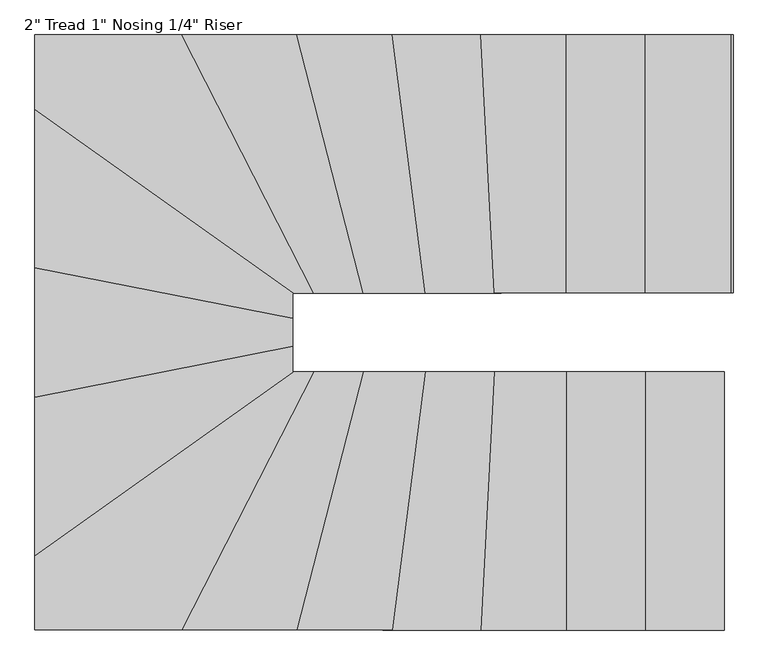
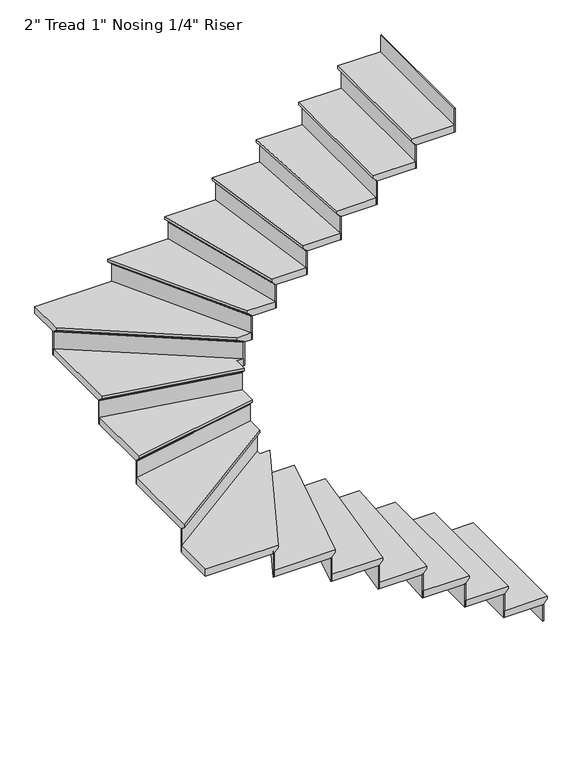
"""IFC4 building model written with IfcOpenShell, lengths in millimetres: stair flight geometry."""

from ifc_helpers import new_model, si_unit, origin, place, context, project, spatial, faceted_brep, source, transform, mapped, element, save


def stair_flight_a924437b(model_context):
    return source(origin(), model_context, "Body", "Brep", [
        faceted_brep([(-7708.0614906, -9206.110779, 6863.0131579), (-7708.0614906, -9206.110779, 6882.0631579), (-7708.0614906, -10120.510779, 6882.0631579), (-7708.0614906, -10120.510779, 6863.0131579), (-7733.4614906, -9206.110779, 6837.6131579), (-7733.4614906, -10120.510779, 6837.6131579), (-8012.8614906, -9206.110779, 6882.0631579), (-8012.8614906, -10120.510779, 6882.0631579), (-7733.4614906, -10120.510779, 6831.2631579), (-8012.8614906, -10120.510779, 6831.2631579), (-8012.8614906, -9206.110779, 6831.2631579), (-7733.4614906, -9206.110779, 6831.2631579)], [[[0, 1, 2, 3]], [[4, 0, 3, 5]], [[2, 1, 6, 7]], [[8, 9, 10, 11]], [[2, 7, 9, 8, 5, 3]], [[8, 11, 4, 5]], [[6, 1, 0, 4, 11, 10]], [[7, 6, 10, 9]]]),
        faceted_brep([(-7733.4614906, -9206.110779, 6831.2631579), (-7733.4614906, -9206.110779, 6705.6), (-7739.8114906, -9206.110779, 6705.6), (-7739.8114906, -9206.110779, 6831.2631579), (-7733.4614906, -10120.510779, 6831.2631579), (-7739.8114906, -10120.510779, 6831.2631579), (-7739.8114906, -10120.510779, 6705.6), (-7733.4614906, -10120.510779, 6705.6)], [[[0, 1, 2, 3]], [[4, 5, 6, 7]], [[1, 0, 4, 7]], [[2, 1, 7, 6]], [[3, 2, 6, 5]], [[0, 3, 5, 4]]]),
        faceted_brep([(-8012.8614906, -9206.110779, 7007.7263158), (-8012.8614906, -9206.110779, 6831.2631579), (-8019.2114906, -9206.110779, 6831.2631579), (-8019.2114906, -9206.110779, 7007.7263158), (-8012.8614906, -10120.510779, 7007.7263158), (-8019.2114906, -10120.510779, 7007.7263158), (-8019.2114906, -10120.510779, 6831.2631579), (-8012.8614906, -10120.510779, 6831.2631579)], [[[0, 1, 2, 3]], [[4, 5, 6, 7]], [[1, 0, 4, 7]], [[2, 1, 7, 6]], [[3, 2, 6, 5]], [[0, 3, 5, 4]]]),
        faceted_brep([(-7987.4614906, -10120.510779, 7058.5263158), (-7987.4614906, -9206.110779, 7058.5263158), (-8292.2614906, -9206.110779, 7058.5263158), (-8292.2614906, -10120.510779, 7058.5263158), (-8012.8614906, -10120.510779, 7007.7263158), (-8292.2614906, -10120.510779, 7007.7263158), (-8292.2614906, -9206.110779, 7007.7263158), (-8012.8614906, -9206.110779, 7007.7263158), (-8012.8614906, -10120.510779, 7014.0763158), (-7987.4614906, -10120.510779, 7039.4763158), (-8012.8614906, -9206.110779, 7014.0763158), (-7987.4614906, -9206.110779, 7039.4763158)], [[[0, 1, 2, 3]], [[4, 5, 6, 7]], [[0, 3, 5, 4, 8, 9]], [[4, 7, 10, 8]], [[2, 1, 11, 10, 7, 6]], [[3, 2, 6, 5]], [[11, 1, 0, 9]], [[10, 11, 9, 8]]]),
        faceted_brep([(-8292.2614906, -9206.110779, 7184.1894737), (-8292.2614906, -9206.110779, 7007.7263158), (-8298.6114906, -9206.110779, 7007.7263158), (-8298.6114906, -9206.110779, 7184.1894737), (-8292.2614906, -10120.510779, 7184.1894737), (-8298.6114906, -10120.510779, 7184.1894737), (-8298.6114906, -10120.510779, 7007.7263158), (-8292.2614906, -10120.510779, 7007.7263158)], [[[0, 1, 2, 3]], [[4, 5, 6, 7]], [[1, 0, 4, 7]], [[2, 1, 7, 6]], [[3, 2, 6, 5]], [[0, 3, 5, 4]]]),
        faceted_brep([(-8266.8614906, -10120.510779, 7234.9894737), (-8266.8614906, -9206.110779, 7234.9894737), (-8547.928652, -9206.110779, 7234.9894737), (-8595.4629224, -10120.510779, 7234.9894737), (-8292.2614906, -10120.510779, 7184.1894737), (-8595.4629224, -10120.510779, 7184.1894737), (-8547.928652, -9206.110779, 7184.1894737), (-8292.2614906, -9206.110779, 7184.1894737), (-8292.2614906, -10120.510779, 7190.5394737), (-8266.8614906, -10120.510779, 7215.9394737), (-8292.2614906, -9206.110779, 7190.5394737), (-8266.8614906, -9206.110779, 7215.9394737)], [[[0, 1, 2, 3]], [[4, 5, 6, 7]], [[0, 3, 5, 4, 8, 9]], [[4, 7, 10, 8]], [[2, 1, 11, 10, 7, 6]], [[3, 2, 6, 5]], [[11, 1, 0, 9]], [[10, 11, 9, 8]]]),
        faceted_brep([(-8547.928652, -9206.110779, 7360.6526316), (-8547.928652, -9206.110779, 7184.1894737), (-8554.2872262, -9206.110779, 7184.1894737), (-8554.2872262, -9206.110779, 7360.6526316), (-8595.4629224, -10120.510779, 7360.6526316), (-8601.8214966, -10120.510779, 7360.6526316), (-8601.8214966, -10120.510779, 7184.1894737), (-8595.4629224, -10120.510779, 7184.1894737)], [[[0, 1, 2, 3]], [[4, 5, 6, 7]], [[1, 0, 4, 7]], [[2, 1, 7, 6]], [[3, 2, 6, 5]], [[0, 3, 5, 4]]]),
        faceted_brep([(-8570.0286258, -10120.510779, 7411.4526316), (-8522.4943554, -9206.110779, 7411.4526316), (-8792.0953519, -9206.110779, 7411.4526316), (-8910.4514035, -10120.510779, 7411.4526316), (-8595.4629224, -10120.510779, 7360.6526316), (-8910.4514035, -10120.510779, 7360.6526316), (-8792.0953519, -9206.110779, 7360.6526316), (-8547.928652, -9206.110779, 7360.6526316), (-8595.4629224, -10120.510779, 7367.0026316), (-8570.0286258, -10120.510779, 7392.4026316), (-8547.928652, -9206.110779, 7367.0026316), (-8522.4943554, -9206.110779, 7392.4026316)], [[[0, 1, 2, 3]], [[4, 5, 6, 7]], [[0, 3, 5, 4, 8, 9]], [[4, 7, 10, 8]], [[2, 1, 11, 10, 7, 6]], [[3, 2, 6, 5]], [[11, 1, 0, 9]], [[10, 11, 9, 8]]]),
        faceted_brep([(-8792.0953519, -9206.110779, 7537.1157895), (-8792.0953519, -9206.110779, 7360.6526316), (-8798.4983236, -9206.110779, 7360.6526316), (-8798.4983236, -9206.110779, 7537.1157895), (-8910.4514035, -10120.510779, 7537.1157895), (-8916.8543753, -10120.510779, 7537.1157895), (-8916.8543753, -10120.510779, 7360.6526316), (-8910.4514035, -10120.510779, 7360.6526316)], [[[0, 1, 2, 3]], [[4, 5, 6, 7]], [[1, 0, 4, 7]], [[2, 1, 7, 6]], [[3, 2, 6, 5]], [[0, 3, 5, 4]]]),
        faceted_brep([(-8884.8395164, -10120.510779, 7587.9157895), (-8766.4834647, -9206.110779, 7587.9157895), (-9013.7225743, -9206.110779, 7587.9157895), (-9248.8530217, -10120.510779, 7587.9157895), (-8910.4514035, -10120.510779, 7537.1157895), (-9248.8530217, -10120.510779, 7537.1157895), (-9013.7225743, -9206.110779, 7537.1157895), (-8792.0953519, -9206.110779, 7537.1157895), (-8910.4514035, -10120.510779, 7543.4657895), (-8884.8395164, -10120.510779, 7568.8657895), (-8792.0953519, -9206.110779, 7543.4657895), (-8766.4834647, -9206.110779, 7568.8657895)], [[[0, 1, 2, 3]], [[4, 5, 6, 7]], [[0, 3, 5, 4, 8, 9]], [[4, 7, 10, 8]], [[2, 1, 11, 10, 7, 6]], [[3, 2, 6, 5]], [[11, 1, 0, 9]], [[10, 11, 9, 8]]]),
        faceted_brep([(-9013.7225743, -9206.110779, 7713.5789474), (-9013.7225743, -9206.110779, 7537.1157895), (-9020.2791512, -9206.110779, 7537.1157895), (-9020.2791512, -9206.110779, 7713.5789474), (-9248.8530217, -10120.510779, 7713.5789474), (-9255.4095986, -10120.510779, 7713.5789474), (-9255.4095986, -10120.510779, 7537.1157895), (-9248.8530217, -10120.510779, 7537.1157895)], [[[0, 1, 2, 3]], [[4, 5, 6, 7]], [[1, 0, 4, 7]], [[2, 1, 7, 6]], [[3, 2, 6, 5]], [[0, 3, 5, 4]]]),
        faceted_brep([(-9222.6267143, -10120.510779, 7764.3789474), (-8987.4962669, -9206.110779, 7764.3789474), (-9190.0692104, -9206.110779, 7764.3789474), (-9658.8938317, -10120.510779, 7764.3789474), (-9248.8530217, -10120.510779, 7713.5789474), (-9658.8938317, -10120.510779, 7713.5789474), (-9190.0692104, -9206.110779, 7713.5789474), (-9013.7225743, -9206.110779, 7713.5789474), (-9248.8530217, -10120.510779, 7719.9289474), (-9222.6267143, -10120.510779, 7745.3289474), (-9013.7225743, -9206.110779, 7719.9289474), (-8987.4962669, -9206.110779, 7745.3289474)], [[[0, 1, 2, 3]], [[4, 5, 6, 7]], [[0, 3, 5, 4, 8, 9]], [[4, 7, 10, 8]], [[2, 1, 11, 10, 7, 6]], [[3, 2, 6, 5]], [[11, 1, 0, 9]], [[10, 11, 9, 8]]]),
        faceted_brep([(-9190.0692104, -9206.110779, 7890.0421053), (-9190.0692104, -9206.110779, 7713.5789474), (-9197.2051936, -9206.110779, 7713.5789474), (-9197.2051936, -9206.110779, 7890.0421053), (-9658.8938317, -10120.510779, 7890.0421053), (-9666.0298149, -10120.510779, 7890.0421053), (-9666.0298149, -10120.510779, 7713.5789474), (-9658.8938317, -10120.510779, 7713.5789474)], [[[0, 1, 2, 3]], [[4, 5, 6, 7]], [[1, 0, 4, 7]], [[2, 1, 7, 6]], [[3, 2, 6, 5]], [[0, 3, 5, 4]]]),
        faceted_brep([(-10150.1931824, -9826.8296453, 7940.8421053), (-10150.1931824, -10120.510779, 7940.8421053), (-9630.3498992, -10120.510779, 7940.8421053), (-9161.5252779, -9206.110779, 7940.8421053), (-9235.7931824, -9206.110779, 7940.8421053), (-9235.7931824, -9176.5556961, 7940.8421053), (-10150.1931824, -10120.510779, 7890.0421053), (-10150.1931824, -9826.8296453, 7890.0421053), (-9235.7931824, -9176.5556961, 7890.0421053), (-9235.7931824, -9206.110779, 7890.0421053), (-9190.0692104, -9206.110779, 7890.0421053), (-9658.8938317, -10120.510779, 7890.0421053), (-9658.8938317, -10120.510779, 7896.3921053), (-9630.3498992, -10120.510779, 7921.7921053), (-9190.0692104, -9206.110779, 7896.3921053), (-9161.5252779, -9206.110779, 7921.7921053)], [[[0, 1, 2, 3, 4, 5]], [[6, 7, 8, 9, 10, 11]], [[1, 0, 7, 6]], [[2, 1, 6, 11, 12, 13]], [[11, 10, 14, 12]], [[4, 3, 15, 14, 10, 9]], [[5, 4, 9, 8]], [[0, 5, 8, 7]], [[15, 3, 2, 13]], [[14, 15, 13, 12]]]),
        faceted_brep([(-9235.7931824, -9176.5556961, 8066.5052632), (-9235.7931824, -9176.5556961, 7890.0421053), (-9235.7931824, -9168.7637213, 7890.0421053), (-9235.7931824, -9168.7637213, 8066.5052632), (-10150.1931824, -9826.8296453, 8066.5052632), (-10150.1931824, -9819.0376705, 8066.5052632), (-10150.1931824, -9819.0376705, 7890.0421053), (-10150.1931824, -9826.8296453, 7890.0421053)], [[[0, 1, 2, 3]], [[4, 5, 6, 7]], [[1, 0, 4, 7]], [[2, 1, 7, 6]], [[3, 2, 6, 5]], [[0, 3, 5, 4]]]),
        faceted_brep([(-10150.1931824, -9857.9975445, 8117.3052632), (-9235.7931824, -9207.7235953, 8117.3052632), (-9235.7931824, -9090.1016091, 8117.3052632), (-10150.1931824, -9270.3424654, 8117.3052632), (-10150.1931824, -9826.8296453, 8066.5052632), (-10150.1931824, -9270.3424654, 8066.5052632), (-9235.7931824, -9090.1016091, 8066.5052632), (-9235.7931824, -9176.5556961, 8066.5052632), (-10150.1931824, -9826.8296453, 8072.8552632), (-10150.1931824, -9857.9975445, 8098.2552632), (-9235.7931824, -9176.5556961, 8072.8552632), (-9235.7931824, -9207.7235953, 8098.2552632)], [[[0, 1, 2, 3]], [[4, 5, 6, 7]], [[0, 3, 5, 4, 8, 9]], [[4, 7, 10, 8]], [[2, 1, 11, 10, 7, 6]], [[3, 2, 6, 5]], [[11, 1, 0, 9]], [[10, 11, 9, 8]]]),
        faceted_brep([(-9235.7931824, -9090.1016091, 8242.9684211), (-9235.7931824, -9090.1016091, 8066.5052632), (-9235.7931824, -9083.6294236, 8066.5052632), (-9235.7931824, -9083.6294236, 8242.9684211), (-10150.1931824, -9270.3424654, 8242.9684211), (-10150.1931824, -9263.87028, 8242.9684211), (-10150.1931824, -9263.87028, 8066.5052632), (-10150.1931824, -9270.3424654, 8066.5052632)], [[[0, 1, 2, 3]], [[4, 5, 6, 7]], [[1, 0, 4, 7]], [[2, 1, 7, 6]], [[3, 2, 6, 5]], [[0, 3, 5, 4]]]),
        faceted_brep([(-10150.1931824, -9296.2312071, 8293.7684211), (-9235.7931824, -9115.9903508, 8293.7684211), (-9235.7931824, -8990.9424654, 8293.7684211), (-10150.1931824, -8810.7016091, 8293.7684211), (-10150.1931824, -9270.3424654, 8242.9684211), (-10150.1931824, -8810.7016091, 8242.9684211), (-9235.7931824, -8990.9424654, 8242.9684211), (-9235.7931824, -9090.1016091, 8242.9684211), (-10150.1931824, -9270.3424654, 8249.3184211), (-10150.1931824, -9296.2312071, 8274.7184211), (-9235.7931824, -9090.1016091, 8249.3184211), (-9235.7931824, -9115.9903508, 8274.7184211)], [[[0, 1, 2, 3]], [[4, 5, 6, 7]], [[0, 3, 5, 4, 8, 9]], [[4, 7, 10, 8]], [[2, 1, 11, 10, 7, 6]], [[3, 2, 6, 5]], [[11, 1, 0, 9]], [[10, 11, 9, 8]]]),
        faceted_brep([(-9235.7931824, -8990.9424654, 8419.4315789), (-9235.7931824, -8990.9424654, 8242.9684211), (-9235.7931824, -8984.47028, 8242.9684211), (-9235.7931824, -8984.47028, 8419.4315789), (-10150.1931824, -8810.7016091, 8419.4315789), (-10150.1931824, -8804.2294236, 8419.4315789), (-10150.1931824, -8804.2294236, 8242.9684211), (-10150.1931824, -8810.7016091, 8242.9684211)], [[[0, 1, 2, 3]], [[4, 5, 6, 7]], [[1, 0, 4, 7]], [[2, 1, 7, 6]], [[3, 2, 6, 5]], [[0, 3, 5, 4]]]),
        faceted_brep([(-10150.1931824, -8836.5903508, 8470.2315789), (-9235.7931824, -9016.8312071, 8470.2315789), (-9235.7931824, -8926.710779, 8470.2315789), (-9189.6977079, -8926.710779, 8470.2315789), (-10150.1931824, -8243.6561143, 8470.2315789), (-10150.1931824, -8810.7016091, 8419.4315789), (-10150.1931824, -8243.6561143, 8419.4315789), (-9189.6977079, -8926.710779, 8419.4315789), (-9235.7931824, -8926.710779, 8419.4315789), (-9235.7931824, -8990.9424654, 8419.4315789), (-10150.1931824, -8810.7016091, 8425.7815789), (-10150.1931824, -8836.5903508, 8451.1815789), (-9235.7931824, -8990.9424654, 8425.7815789), (-9235.7931824, -9016.8312071, 8451.1815789)], [[[0, 1, 2, 3, 4]], [[5, 6, 7, 8, 9]], [[0, 4, 6, 5, 10, 11]], [[5, 9, 12, 10]], [[2, 1, 13, 12, 9, 8]], [[3, 2, 8, 7]], [[4, 3, 7, 6]], [[13, 1, 0, 11]], [[12, 13, 11, 10]]]),
        faceted_brep([(-9189.6977079, -8926.710779, 8595.8947368), (-9189.6977079, -8926.710779, 8419.4315789), (-9178.7408154, -8926.710779, 8419.4315789), (-9178.7408154, -8926.710779, 8595.8947368), (-10150.1931824, -8243.6561143, 8595.8947368), (-10150.1931824, -8235.8641395, 8595.8947368), (-10150.1931824, -8235.8641395, 8419.4315789), (-10150.1931824, -8243.6561143, 8419.4315789)], [[[0, 1, 2, 3]], [[4, 5, 6, 7]], [[1, 0, 4, 7]], [[2, 1, 7, 6]], [[3, 2, 6, 5]], [[0, 3, 5, 4]]]),
        faceted_brep([(-9601.8059667, -8012.310779, 8646.6947368), (-10150.1931824, -8012.310779, 8646.6947368), (-10150.1931824, -8274.8240135, 8646.6947368), (-9233.5252779, -8926.710779, 8646.6947368), (-9132.9813454, -8926.710779, 8646.6947368), (-10150.1931824, -8012.310779, 8595.8947368), (-9601.8059667, -8012.310779, 8595.8947368), (-9132.9813454, -8926.710779, 8595.8947368), (-9189.6977079, -8926.710779, 8595.8947368), (-10150.1931824, -8243.6561143, 8595.8947368), (-10150.1931824, -8243.6561143, 8602.2447368), (-10150.1931824, -8274.8240135, 8627.6447368), (-9189.6977079, -8926.710779, 8602.2447368), (-9233.5252779, -8926.710779, 8627.6447368)], [[[0, 1, 2, 3, 4]], [[5, 6, 7, 8, 9]], [[1, 0, 6, 5]], [[2, 1, 5, 9, 10, 11]], [[9, 8, 12, 10]], [[4, 3, 13, 12, 8, 7]], [[0, 4, 7, 6]], [[13, 3, 2, 11]], [[12, 13, 11, 10]]]),
        faceted_brep([(-9132.9813454, -8926.710779, 8772.3578947), (-9132.9813454, -8926.710779, 8595.8947368), (-9125.8453622, -8926.710779, 8595.8947368), (-9125.8453622, -8926.710779, 8772.3578947), (-9601.8059667, -8012.310779, 8772.3578947), (-9594.6699835, -8012.310779, 8772.3578947), (-9594.6699835, -8012.310779, 8595.8947368), (-9601.8059667, -8012.310779, 8595.8947368)], [[[0, 1, 2, 3]], [[4, 5, 6, 7]], [[1, 0, 4, 7]], [[2, 1, 7, 6]], [[3, 2, 6, 5]], [[0, 3, 5, 4]]]),
        faceted_brep([(-9630.3498992, -8012.310779, 8823.1578947), (-9161.5252779, -8926.710779, 8823.1578947), (-8961.2699594, -8926.710779, 8823.1578947), (-9196.4004068, -8012.310779, 8823.1578947), (-9601.8059667, -8012.310779, 8772.3578947), (-9196.4004068, -8012.310779, 8772.3578947), (-8961.2699594, -8926.710779, 8772.3578947), (-9132.9813454, -8926.710779, 8772.3578947), (-9601.8059667, -8012.310779, 8778.7078947), (-9630.3498992, -8012.310779, 8804.1078947), (-9132.9813454, -8926.710779, 8778.7078947), (-9161.5252779, -8926.710779, 8804.1078947)], [[[0, 1, 2, 3]], [[4, 5, 6, 7]], [[0, 3, 5, 4, 8, 9]], [[4, 7, 10, 8]], [[2, 1, 11, 10, 7, 6]], [[3, 2, 6, 5]], [[11, 1, 0, 9]], [[10, 11, 9, 8]]]),
        faceted_brep([(-8961.2699594, -8926.710779, 8948.8210526), (-8961.2699594, -8926.710779, 8772.3578947), (-8954.7133825, -8926.710779, 8772.3578947), (-8954.7133825, -8926.710779, 8948.8210526), (-9196.4004068, -8012.310779, 8948.8210526), (-9189.84383, -8012.310779, 8948.8210526), (-9189.84383, -8012.310779, 8772.3578947), (-9196.4004068, -8012.310779, 8772.3578947)], [[[0, 1, 2, 3]], [[4, 5, 6, 7]], [[1, 0, 4, 7]], [[2, 1, 7, 6]], [[3, 2, 6, 5]], [[0, 3, 5, 4]]]),
        faceted_brep([(-9222.6267143, -8012.310779, 8999.6210526), (-8987.4962669, -8926.710779, 8999.6210526), (-8740.8715776, -8926.710779, 8999.6210526), (-8859.2276293, -8012.310779, 8999.6210526), (-9196.4004068, -8012.310779, 8948.8210526), (-8859.2276293, -8012.310779, 8948.8210526), (-8740.8715776, -8926.710779, 8948.8210526), (-8961.2699594, -8926.710779, 8948.8210526), (-9196.4004068, -8012.310779, 8955.1710526), (-9222.6267143, -8012.310779, 8980.5710526), (-8961.2699594, -8926.710779, 8955.1710526), (-8987.4962669, -8926.710779, 8980.5710526)], [[[0, 1, 2, 3]], [[4, 5, 6, 7]], [[0, 3, 5, 4, 8, 9]], [[4, 7, 10, 8]], [[2, 1, 11, 10, 7, 6]], [[3, 2, 6, 5]], [[11, 1, 0, 9]], [[10, 11, 9, 8]]]),
        faceted_brep([(-8740.8715776, -8926.710779, 9125.2842105), (-8740.8715776, -8926.710779, 8948.8210526), (-8734.4686059, -8926.710779, 8948.8210526), (-8734.4686059, -8926.710779, 9125.2842105), (-8859.2276293, -8012.310779, 9125.2842105), (-8852.8246575, -8012.310779, 9125.2842105), (-8852.8246575, -8012.310779, 8948.8210526), (-8859.2276293, -8012.310779, 8948.8210526)], [[[0, 1, 2, 3]], [[4, 5, 6, 7]], [[1, 0, 4, 7]], [[2, 1, 7, 6]], [[3, 2, 6, 5]], [[0, 3, 5, 4]]]),
        faceted_brep([(-8884.8395164, -8012.310779, 9176.0842105), (-8766.4834647, -8926.710779, 9176.0842105), (-8497.0600587, -8926.710779, 9176.0842105), (-8544.5943291, -8012.310779, 9176.0842105), (-8859.2276293, -8012.310779, 9125.2842105), (-8544.5943291, -8012.310779, 9125.2842105), (-8497.0600587, -8926.710779, 9125.2842105), (-8740.8715776, -8926.710779, 9125.2842105), (-8859.2276293, -8012.310779, 9131.6342105), (-8884.8395164, -8012.310779, 9157.0342105), (-8740.8715776, -8926.710779, 9131.6342105), (-8766.4834647, -8926.710779, 9157.0342105)], [[[0, 1, 2, 3]], [[4, 5, 6, 7]], [[0, 3, 5, 4, 8, 9]], [[4, 7, 10, 8]], [[2, 1, 11, 10, 7, 6]], [[3, 2, 6, 5]], [[11, 1, 0, 9]], [[10, 11, 9, 8]]]),
        faceted_brep([(-8497.0600587, -8926.710779, 9301.7473684), (-8497.0600587, -8926.710779, 9125.2842105), (-8490.7014845, -8926.710779, 9125.2842105), (-8490.7014845, -8926.710779, 9301.7473684), (-8544.5943291, -8012.310779, 9301.7473684), (-8538.235755, -8012.310779, 9301.7473684), (-8538.235755, -8012.310779, 9125.2842105), (-8544.5943291, -8012.310779, 9125.2842105)], [[[0, 1, 2, 3]], [[4, 5, 6, 7]], [[1, 0, 4, 7]], [[2, 1, 7, 6]], [[3, 2, 6, 5]], [[0, 3, 5, 4]]]),
        faceted_brep([(-8570.0286258, -8012.310779, 9352.5473684), (-8522.4943554, -8926.710779, 9352.5473684), (-8241.4614906, -8926.710779, 9352.5473684), (-8241.4614906, -8012.310779, 9352.5473684), (-8544.5943291, -8012.310779, 9301.7473684), (-8241.4614906, -8012.310779, 9301.7473684), (-8241.4614906, -8926.710779, 9301.7473684), (-8497.0600587, -8926.710779, 9301.7473684), (-8544.5943291, -8012.310779, 9308.0973684), (-8570.0286258, -8012.310779, 9333.4973684), (-8497.0600587, -8926.710779, 9308.0973684), (-8522.4943554, -8926.710779, 9333.4973684)], [[[0, 1, 2, 3]], [[4, 5, 6, 7]], [[0, 3, 5, 4, 8, 9]], [[4, 7, 10, 8]], [[2, 1, 11, 10, 7, 6]], [[3, 2, 6, 5]], [[11, 1, 0, 9]], [[10, 11, 9, 8]]]),
        faceted_brep([(-8241.4614906, -8926.710779, 9478.2105263), (-8241.4614906, -8926.710779, 9301.7473684), (-8235.1114906, -8926.710779, 9301.7473684), (-8235.1114906, -8926.710779, 9478.2105263), (-8241.4614906, -8012.310779, 9478.2105263), (-8235.1114906, -8012.310779, 9478.2105263), (-8235.1114906, -8012.310779, 9301.7473684), (-8241.4614906, -8012.310779, 9301.7473684)], [[[0, 1, 2, 3]], [[4, 5, 6, 7]], [[1, 0, 4, 7]], [[2, 1, 7, 6]], [[3, 2, 6, 5]], [[0, 3, 5, 4]]]),
        faceted_brep([(-8266.8614906, -8012.310779, 9529.0105263), (-8266.8614906, -8926.710779, 9529.0105263), (-7962.0614906, -8926.710779, 9529.0105263), (-7962.0614906, -8012.310779, 9529.0105263), (-8241.4614906, -8012.310779, 9478.2105263), (-7962.0614906, -8012.310779, 9478.2105263), (-7962.0614906, -8926.710779, 9478.2105263), (-8241.4614906, -8926.710779, 9478.2105263), (-8241.4614906, -8012.310779, 9484.5605263), (-8266.8614906, -8012.310779, 9509.9605263), (-8241.4614906, -8926.710779, 9484.5605263), (-8266.8614906, -8926.710779, 9509.9605263)], [[[0, 1, 2, 3]], [[4, 5, 6, 7]], [[0, 3, 5, 4, 8, 9]], [[4, 7, 10, 8]], [[2, 1, 11, 10, 7, 6]], [[3, 2, 6, 5]], [[11, 1, 0, 9]], [[10, 11, 9, 8]]]),
        faceted_brep([(-7962.0614906, -8926.710779, 9654.6736842), (-7962.0614906, -8926.710779, 9478.2105263), (-7955.7114906, -8926.710779, 9478.2105263), (-7955.7114906, -8926.710779, 9654.6736842), (-7962.0614906, -8012.310779, 9654.6736842), (-7955.7114906, -8012.310779, 9654.6736842), (-7955.7114906, -8012.310779, 9478.2105263), (-7962.0614906, -8012.310779, 9478.2105263)], [[[0, 1, 2, 3]], [[4, 5, 6, 7]], [[1, 0, 4, 7]], [[2, 1, 7, 6]], [[3, 2, 6, 5]], [[0, 3, 5, 4]]]),
        faceted_brep([(-7682.6614906, -8926.710779, 9831.1368421), (-7682.6614906, -8926.710779, 9654.6736842), (-7676.3114906, -8926.710779, 9654.6736842), (-7676.3114906, -8926.710779, 9831.1368421), (-7682.6614906, -8012.310779, 9831.1368421), (-7676.3114906, -8012.310779, 9831.1368421), (-7676.3114906, -8012.310779, 9654.6736842), (-7682.6614906, -8012.310779, 9654.6736842)], [[[0, 1, 2, 3]], [[4, 5, 6, 7]], [[1, 0, 4, 7]], [[2, 1, 7, 6]], [[3, 2, 6, 5]], [[0, 3, 5, 4]]]),
        faceted_brep([(-7987.4614906, -8012.310779, 9705.4736842), (-7987.4614906, -8926.710779, 9705.4736842), (-7682.6614906, -8926.710779, 9705.4736842), (-7682.6614906, -8012.310779, 9705.4736842), (-7962.0614906, -8012.310779, 9654.6736842), (-7682.6614906, -8012.310779, 9654.6736842), (-7682.6614906, -8926.710779, 9654.6736842), (-7962.0614906, -8926.710779, 9654.6736842), (-7962.0614906, -8012.310779, 9661.0236842), (-7987.4614906, -8012.310779, 9686.4236842), (-7962.0614906, -8926.710779, 9661.0236842), (-7987.4614906, -8926.710779, 9686.4236842)], [[[0, 1, 2, 3]], [[4, 5, 6, 7]], [[0, 3, 5, 4, 8, 9]], [[4, 7, 10, 8]], [[2, 1, 11, 10, 7, 6]], [[3, 2, 6, 5]], [[11, 1, 0, 9]], [[10, 11, 9, 8]]]),
    ])


if __name__ == "__main__":
    model = new_model("IFC4")
    model_context = context("Model", 3, world=origin())
    ifc_project = project(units=[si_unit("LENGTHUNIT", "METRE", prefix="MILLI")], contexts=[model_context])
    site = spatial("IfcSite", under=ifc_project)
    building = spatial("IfcBuilding", under=site)
    placement = place(None, origin())
    stair_flight_shape = stair_flight_a924437b(model_context)
    element("IfcStairFlight", 1, ObjectType="2\" Tread 1\" Nosing 1/4\" Riser", at=placement, inside=building, context=model_context, shape_type="MappedRepresentation", body=[
        mapped(stair_flight_shape, transform((0.0, 0.0, 0.0), x_axis=(1.0, 0.0, 0.0), y_axis=(0.0, 1.0, 0.0), z_axis=(0.0, 0.0, 1.0))),
    ])
    save(model, "model.ifc")
